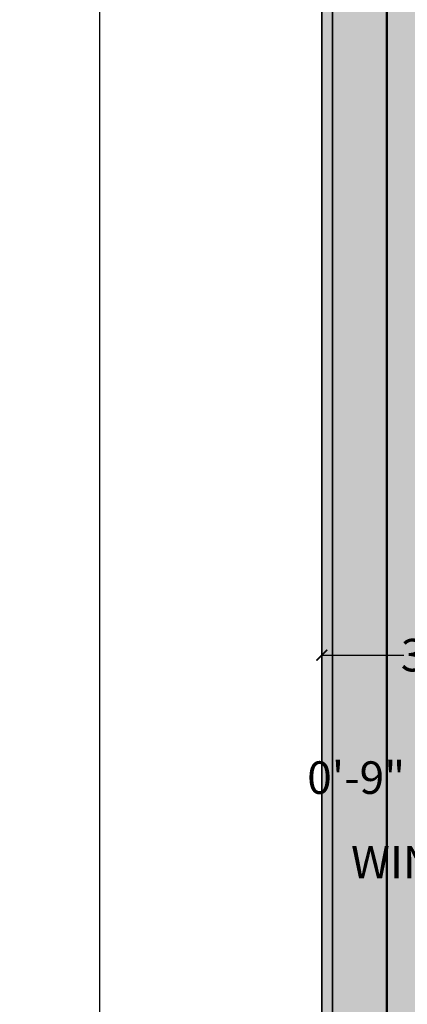
# Model space of a CAD drawing. Units: inches. Extents: x 528 to 2620, y -1066 to 798.
# Tile 5 of 41: x 528 to 600, y 523 to 705. Entities that reach past the tile are written whole.
import ezdxf

# ---------------------------------------------------------------- set-up
doc = ezdxf.new("R2010")
doc.units = ezdxf.units.IN
doc.header["$MEASUREMENT"] = 0
for name, color, linetype, lineweight in [('A-ANNO-DIMS', 2, 'Continuous', 18), ('A-WALL', 7, 'Continuous', 50), ('A-WALL-PATT', 8, 'Continuous', 13), ('C-PROP', 5, 'Continuous', 35)]:
    doc.layers.add(name, color=color, linetype=linetype, lineweight=lineweight)
doc.styles.get("Standard").update_dxf_attribs({"font": 'arial.ttf'})
doc.dimstyles.get("Standard").update_dxf_attribs({"dimtxt": 6, "dimasz": 2, "dimexe": 0.18, "dimexo": 0.0625, "dimgap": 0.09, "dimtad": 0, "dimtih": 1, "dimtoh": 1, "dimdec": 1, "dimzin": 0, "dimdsep": 46, "dimlunit": 3, "dimtxsty": 'Standard', "dimblk": 'ARCHTICK', "dimcen": 0.09, "dimadec": 0, "dimazin": 0, "dimtfac": 1, "dimtdec": 1, "dimtofl": 0, "dimtmove": 0, "dimatfit": 3, "dimfxl": 1, "dimtolj": 1, "dimtzin": 0, "dimarcsym": 0})

# ---------------------------------------------------------------- blocks, each defined once
blk = doc.blocks.new('_ArchTick')
at = {"color": 0, "linetype": 'ByBlock', "const_width": 0.15}
blk.add_lwpolyline([(-0.5, -0.5), (0.5, 0.5)], dxfattribs=at)
blk = doc.blocks.new('*D12')
at = {"layer": 'A-ANNO-DIMS', "color": 0, "lineweight": -2, "transparency": 16777216}
for p, q in [((584, 753.92), (542.88, 753.92)), ((543.06, 753.92), (543.06, 484.58)), ((543.06, 208.92), (543.06, 478.27)), ((584, 208.92), (542.88, 208.92))]:
    blk.add_line(p, q, dxfattribs=at)
at = {"layer": 'Defpoints', "color": 0, "transparency": 16777216}
for p in [(584.06, 753.92), (543.06, 208.92), (584.06, 208.92)]:
    blk.add_point(p, dxfattribs=at)
at = {"layer": 'A-ANNO-DIMS', "color": 0, "lineweight": -2, "transparency": 16777216, "xscale": 2, "yscale": 2, "zscale": 2}
for p, rotation in [((543.06, 753.92), 90), ((543.06, 208.92), 270)]:
    blk.add_blockref('_ArchTick', p, dxfattribs=dict(at, rotation=rotation))
at = {"layer": 'A-ANNO-DIMS', "color": 0, "transparency": 16777216, "insert": (543.06, 481.42), "char_height": 6, "attachment_point": 5}
blk.add_mtext('\\A1;45\'-5.0"', dxfattribs=at)
blk = doc.blocks.new('*D14')
at = {"layer": 'A-ANNO-DIMS', "color": 0, "lineweight": -2, "transparency": 16777216}
for p, q in [((584.06, 587.76), (584.06, 587.45)), ((584.06, 587.63), (599.21, 587.63)), ((620.06, 587.63), (604.91, 587.63)), ((620.06, 587.76), (620.06, 587.45))]:
    blk.add_line(p, q, dxfattribs=at)
at = {"layer": 'Defpoints', "color": 0, "transparency": 16777216}
for p in [(584.06, 587.82), (584.06, 587.63), (620.06, 587.82)]:
    blk.add_point(p, dxfattribs=at)
at = {"layer": 'A-ANNO-DIMS', "color": 0, "lineweight": -2, "transparency": 16777216, "xscale": 2, "yscale": 2, "zscale": 2, "rotation": 180}
blk.add_blockref('_ArchTick', (584.06, 587.63), dxfattribs=at)
at = {"layer": 'A-ANNO-DIMS', "color": 0, "lineweight": -2, "transparency": 16777216, "xscale": 2, "yscale": 2, "zscale": 2}
blk.add_blockref('_ArchTick', (620.06, 587.63), dxfattribs=at)
at = {"layer": 'A-ANNO-DIMS', "color": 0, "transparency": 16777216, "insert": (602.06, 587.63), "char_height": 6, "attachment_point": 5}
blk.add_mtext("\\A1;3'", dxfattribs=at)
blk = doc.blocks.new('*D52')
at = {"layer": 'A-ANNO-DIMS', "color": 0, "lineweight": -2, "transparency": 16777216}
for p, q in [((629.12, 561.42), (632.84, 561.42)), ((632.66, 561.42), (632.66, 552.62)), ((632.66, 537.42), (632.66, 546.23)), ((629.12, 537.42), (632.84, 537.42))]:
    blk.add_line(p, q, dxfattribs=at)
at = {"layer": 'Defpoints', "color": 0, "transparency": 16777216}
for p in [(629.06, 561.42), (632.66, 561.42), (629.06, 537.42)]:
    blk.add_point(p, dxfattribs=at)
at = {"layer": 'A-ANNO-DIMS', "color": 0, "lineweight": -2, "transparency": 16777216, "xscale": 2, "yscale": 2, "zscale": 2}
for p, rotation in [((632.66, 561.42), 90), ((632.66, 537.42), 270)]:
    blk.add_blockref('_ArchTick', p, dxfattribs=dict(at, rotation=rotation))
at = {"layer": 'A-ANNO-DIMS', "color": 0, "transparency": 16777216, "insert": (632.66, 549.42), "char_height": 6, "attachment_point": 5}
blk.add_mtext('\\A1;WINDOW W2 2\'-0" TYP.', dxfattribs=at)
blk = doc.blocks.new('*D53')
at = {"layer": 'A-ANNO-DIMS', "color": 0, "lineweight": -2, "transparency": 16777216}
for p, q in [((620.06, 565.02), (618.06, 565.02)), ((620.06, 561.48), (620.06, 565.2)), ((629.06, 565.02), (620.06, 565.02)), ((629.06, 561.48), (629.06, 565.2))]:
    blk.add_line(p, q, dxfattribs=at)
at = {"layer": 'Defpoints', "color": 0, "transparency": 16777216}
for p in [(620.06, 565.02), (620.06, 561.42), (629.06, 561.42)]:
    blk.add_point(p, dxfattribs=at)
at = {"layer": 'A-ANNO-DIMS', "color": 0, "lineweight": -2, "transparency": 16777216, "xscale": 2, "yscale": 2, "zscale": 2, "rotation": 180}
blk.add_blockref('_ArchTick', (620.06, 565.02), dxfattribs=at)
at = {"layer": 'A-ANNO-DIMS', "color": 0, "lineweight": -2, "transparency": 16777216, "xscale": 2, "yscale": 2, "zscale": 2}
blk.add_blockref('_ArchTick', (629.06, 565.02), dxfattribs=at)
at = {"layer": 'A-ANNO-DIMS', "color": 0, "transparency": 16777216, "insert": (599.68, 565.02), "char_height": 6, "attachment_point": 5}
blk.add_mtext('\\A1;0\'-9" TYP.', dxfattribs=at)

msp = doc.modelspace()

# ---------------------------------------------------------------- hatches: boundary and pattern name
at = {"layer": 'A-WALL-PATT', "transparency": 33554687}
h = msp.add_hatch(color=256, dxfattribs=at)
h.dxf.hatch_style = 1
h.paths.add_polyline_path([(944.06, 753.92), (584.06, 753.92), (584.06, 208.92), (608.06, 208.92), (608.06, 210.92), (586.06, 210.92), (586.06, 751.92), (942.06, 751.92), (942.06, 210.92), (728.06, 210.92), (728.06, 208.92), (944.06, 208.92)])
h = msp.add_hatch(color=256, dxfattribs=at)
h.dxf.hatch_style = 1
h.paths.add_polyline_path([(942.06, 751.92), (586.06, 751.92), (586.06, 210.92), (608.06, 210.92), (608.06, 220.92), (596.06, 220.92), (596.06, 741.92), (932.06, 741.92), (932.06, 220.92), (770.06, 220.92), (728.06, 220.92), (728.06, 210.92), (942.06, 210.92)])
at = {"layer": 'A-WALL-PATT', "transparency": 33554475}
h = msp.add_hatch(color=256, dxfattribs=at)
h.dxf.hatch_style = 1
h.paths.add_polyline_path([(620.06, 718.92), (908.06, 718.92), (908.06, 268.92), (770.06, 268.92), (770.06, 220.92), (932.06, 220.92), (932.06, 741.92), (596.06, 741.92), (596.06, 391.42), (620.06, 391.42)])

# ---------------------------------------------------------------- linework, layer by layer
at = {"layer": 'A-WALL'}
msp.add_line((596.06, 741.92), (596.06, 391.42), dxfattribs=at)
at = {"layer": 'C-PROP'}
for points in [[(728.06, 208.92), (944.06, 208.92), (944.06, 753.92), (584.06, 753.92), (584.06, 208.92), (608.06, 208.92)], [(728.06, 210.92), (942.06, 210.92), (942.06, 751.92), (586.06, 751.92), (586.06, 210.92), (608.06, 210.92)]]:
    msp.add_lwpolyline(points, dxfattribs=at)
msp.add_lwpolyline([(596.06, 741.92), (596.06, 220.92), (932.06, 220.92), (932.06, 741.92)], close=True, dxfattribs=at)

# ---------------------------------------------------------------- dimensions: what is measured, and where the dimension line sits
at = {"layer": 'A-ANNO-DIMS'}
dim = msp.add_linear_dim(base=(543.06, 208.92), p1=(584.06, 753.92), p2=(584.06, 208.92), angle=90, dimstyle='Standard', override={"dimclrd": 0, "dimclre": 0, "dimclrt": 0}, dxfattribs=at)
dim.commit()
dim.dimension.update_dxf_attribs({"geometry": '*D12', "text_midpoint": (543.06, 481.42)})
dim = msp.add_linear_dim(base=(584.06, 587.63), p1=(620.06, 587.82), p2=(584.06, 587.82), dimstyle='Standard', override={"dimclrd": 0, "dimclre": 0, "dimclrt": 0}, dxfattribs=at)
dim.commit()
dim.dimension.update_dxf_attribs({"geometry": '*D14', "text_midpoint": (602.06, 587.63)})
for base, p1, p2, angle, text, picture, middle in [((620.06, 565.02), (629.06, 561.42), (620.06, 561.42), 180, '<> TYP.', '*D53', (599.68, 565.02)), ((632.66, 561.42), (629.06, 537.42), (629.06, 561.42), 90, 'WINDOW W2 <> TYP.', '*D52', (632.66, 549.42))]:
    dim = msp.add_linear_dim(base=base, p1=p1, p2=p2, angle=angle, text=text, dimstyle='Standard', override={"dimdec": 1, "dimrnd": 0, "dimzin": 1, "dimlunit": 4, "dimfrac": 2}, dxfattribs=at)
    dim.commit()
    dim.dimension.update_dxf_attribs({"geometry": picture, "text_midpoint": middle})

doc.saveas('drawing.dxf')
